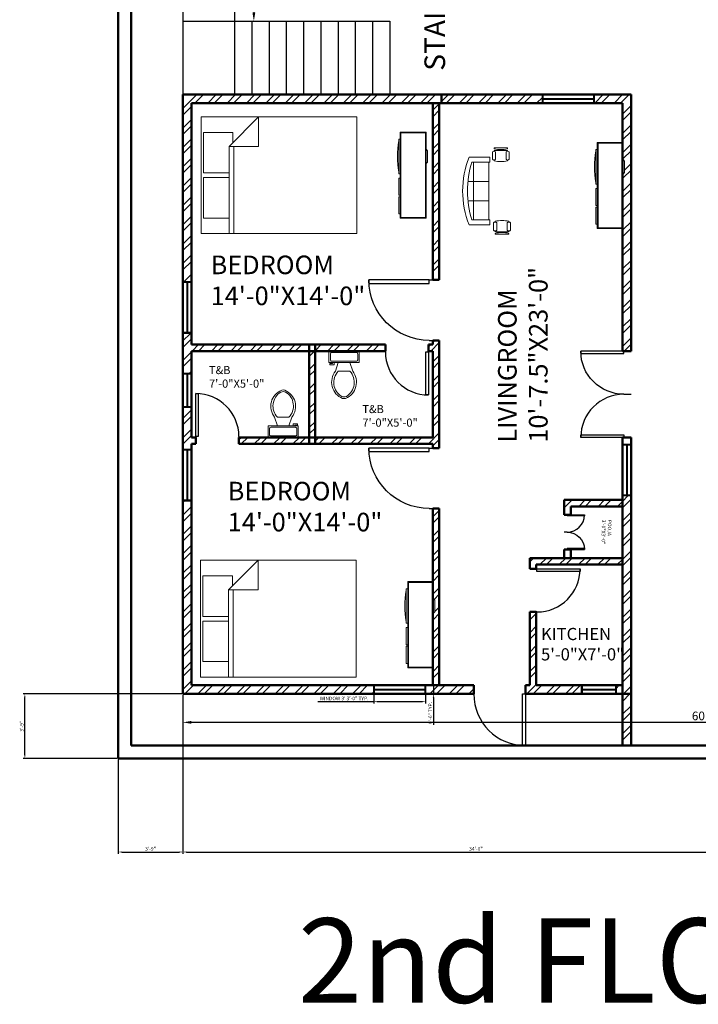
# Model space of a CAD drawing. Units: inches. Extents: x -12550 to 6516, y 1273 to 18700.
# Tile 8 of 19: x 3066 to 3538, y 1273 to 1958. Entities that reach past the tile are written whole.
import ezdxf

# ---------------------------------------------------------------- set-up
doc = ezdxf.new("R2010")
doc.units = ezdxf.units.IN
for name, color, linetype, lineweight in [('A-ANNO-DIMS', 2, 'Continuous', 18), ('A-ANNO-TEXT', 7, 'Continuous', 25), ('A-AREA-IDEN', 1, 'Continuous', 18), ('A-DOOR', 5, 'Continuous', 25), ('A-FLOR-STRS', 6, 'Continuous', 25), ('A-FURN', 8, 'Continuous', 18), ('A-GLAZ', 3, 'Continuous', 25), ('A-WALL', 7, 'Continuous', 50), ('A-WALL-PATT', 8, 'Continuous', 13)]:
    doc.layers.add(name, color=color, linetype=linetype, lineweight=lineweight)
doc.styles.get("Standard").update_dxf_attribs({"font": 'arial.ttf'})
doc.dimstyles.new('ISO-25', dxfattribs={"dimtxt": 2.5, "dimasz": 2.5, "dimexe": 1.25, "dimexo": 0.625, "dimtad": 1, "dimlunit": 4, "dimtxsty": 'Standard', "dimcen": 2.5, "dimadec": 0, "dimazin": 0, "dimtfac": 1, "dimtmove": 0, "dimatfit": 3, "dimfxl": 1, "dimarcsym": 0})
pattern_1 = [(45, (1161.5385, 0), (-6.735192, 6.735192), []), (45, (1166.029, 0), (-6.735192, 6.735192), [])]

# ---------------------------------------------------------------- blocks, each defined once
blk = doc.blocks.new('*U2')
for p, q in [((0, 0), (0, -5)), ((30, 0), (30, -5))]:
    blk.add_line(p, q)
blk.add_lwpolyline([(0, 0), (0, 30), (1.75, 30), (1.75, 0)], close=True)
blk.add_arc((0, 0), 30, 0, 90)
blk = doc.blocks.new('Bed - Queen')
for p, q in [((0, -80.00003), (0, 0)), ((0, 0), (59.99999, 0)), ((59.99999, 0), (59.99999, -80.00003)), ((7.99999, -1.2), (28.79998, -1.2)), ((7.99999, -14.4), (7.99999, -1.2)), ((28.79998, -1.2), (28.79998, -14.4)), ((31.19999, -1.2), (51.99999, -1.2)), ((31.19999, -14.4), (31.19999, -1.2)), ((51.99999, -1.2), (51.99999, -16.4)), ((0, -14.4), (44.8, -14.4)), ((59.99999, -29.6), (44.8, -14.4)), ((44.8, -14.4), (44.8, -29.6)), ((44.8, -16.8), (0, -16.8)), ((51.99999, -16.4), (46.79936, -16.4)), ((44.8, -29.6), (59.99999, -29.6)), ((59.99999, -80.00003), (0, -80.00003))]:
    blk.add_line(p, q)
blk = doc.blocks.new('Toilet - top')
for p, q in [((9.5, -6), (9.5, -2)), ((-10, -8.5), (-8, -8.5)), ((-10, -9.5), (-10, -8.5)), ((-7, -9.5), (-10, -9.5)), ((-8, -8.5), (-8, -8)), ((-7, -8), (-7, -9.5)), ((-4, -8), (-6, -14)), ((4, -8), (6, -14)), ((4, -14), (-4, -14))]:
    blk.add_line(p, q)
blk.add_lwpolyline([(10.5, -8), (10.5, 0), (-10.5, 0), (-10.5, -8)], close=True)
for points in [[(-9.5, -2), (-9.5, -6)], [(8.5, -1), (-8.5, -1)], [(-8.5, -7), (8.5, -7)]]:
    blk.add_lwpolyline(points)
for centre, radius, start, end in [((-8.62, -1.88), 0.884, 81.8699, 188.1301), ((-8.62, -6.12), 0.884, 171.8699, 278.1301), ((8.62, -1.88), 0.884, 351.8699, 98.1301), ((8.62, -6.12), 0.884, 261.8699, 8.1301), ((3.52, -21.58), 12.17, 141.46911, 247.97143), ((4.2, -21.82), 11.33, 136.36773, 238.94682), ((-3.52, -21.58), 12.17, 292.02843, 38.53071), ((-4.2, -21.82), 11.33, 301.05301, 43.63209), ((0, -27.88), 4, 245.73182, 294.26817), ((0, -29), 4, 254.86053, 285.13947)]:
    blk.add_arc(centre, radius, start, end)
blk = doc.blocks.new('Entertainment Center')
for p, q in [((-4, 0), (-5, -1)), ((4, 0), (-4, 0)), ((5, -1), (4, 0)), ((-17, -19), (-17, -1)), ((-17, -1), (43, -1)), ((-16.5, -18.5), (-16.5, -1.5)), ((-16.5, -1.5), (42.5, -1.5)), ((42.5, -1.5), (42.5, -18.5)), ((43, -1), (43, -19)), ((43, -19), (-17, -19)), ((42.5, -18.5), (-16.5, -18.5)), ((-12, -20), (-12, -19)), ((12, -20), (-12, -20)), ((12, -19), (12, -20)), ((15, -20), (15, -19)), ((27, -20), (15, -20)), ((27, -19), (27, -20)), ((28, -20), (28, -19)), ((40, -20), (28, -20)), ((40, -19), (40, -20))]:
    blk.add_line(p, q)
blk.add_arc((0, 40), 61, 259.6111, 280.3889)
blk = doc.blocks.new('Sofa - Roundback 7 ft.')
for p, q in [((-36.000027, -34), (-36.000027, -11.4696)), ((-12.00002, -32.4421), (-12.00003, -6.5971)), ((11.99997, -32.4421), (11.99998, -6.5971)), ((35.99998, -34), (35.99998, -11.4696)), ((-35.999844, -13.3819), (35.9998, -13.3819)), ((-36.000027, -32.4421), (35.99998, -32.4421))]:
    blk.add_line(p, q)
for points in [[(-36.000027, -34), (-42.000027, -34), (-42.000027, -8)], [(41.99998, -8), (41.99998, -34), (35.99998, -34)]]:
    blk.add_lwpolyline(points)
for centre, radius, start, end in [((0, -114.25), 114.25, 68.43141, 111.5686), ((-0.00001, -127.1968), 121.1968, 72.72033, 107.2797)]:
    blk.add_arc(centre, radius, start, end)
blk = doc.blocks.new('Chair - Desk')
for p, q in [((-8.5, 0), (-8.5, -1)), ((-8.5, 0), (8.5, 0)), ((8.5, 0), (8.5, -1)), ((-10.5, -5), (-10.5, -14)), ((-8.5, -3), (-8.5, -4)), ((-8.5, -3), (8.5, -3)), ((-6.5, -14), (-6.5, -5)), ((-2, -3), (-2, -1.9355)), ((2, -1.9576), (2, -3)), ((6.5, -5), (6.5, -14)), ((8.5, -3), (8.5, -4)), ((10.5, -14), (10.5, -5)), ((-8.5, -15), (-8.5, -16)), ((8.5, -15), (8.5, -16))]:
    blk.add_line(p, q)
for centre, radius, start, end in [((-8.5, -6.5), 2.5, 36.8699, 143.1301), ((0, 34.625), 36.625, 256.5803, 283.4197), ((8.5, -6.5), 2.5, 36.8699, 143.1301), ((-8.5, -12.5), 2.5, 216.8699, 323.1301), ((0, 19.625), 36.625, 256.5803, 283.4197), ((8.5, -12.5), 2.5, 216.8699, 323.1301)]:
    blk.add_arc(centre, radius, start, end)
blk = doc.blocks.new('*D36')
at = {"layer": 'A-ANNO-DIMS', "color": 0, "lineweight": -2, "transparency": 16777216}
for p, q in [((3215.85, 2008.25), (3229.9, 2008.25)), ((3228.65, 2002.25), (3228.65, 1963.25)), ((3215.85, 1957.25), (3229.9, 1957.25))]:
    blk.add_line(p, q, dxfattribs=at)
at = {"layer": 'A-ANNO-DIMS', "color": 0, "transparency": 16777216}
for points in [[(3227.65, 2002.25), (3229.65, 2002.25), (3228.65, 2008.25)], [(3227.65, 1963.25), (3229.65, 1963.25), (3228.65, 1957.25)]]:
    blk.add_solid(points, dxfattribs=at)
at = {"layer": 'Defpoints', "color": 0, "transparency": 16777216}
for p in [(3215.23, 2008.25), (3215.23, 1957.25), (3228.65, 1957.25)]:
    blk.add_point(p, dxfattribs=at)
at = {"layer": 'A-ANNO-DIMS', "color": 0, "transparency": 16777216, "insert": (3224.96, 1982.75), "char_height": 6, "attachment_point": 5, "rotation": 90}
blk.add_mtext('4\'-3"', dxfattribs=at)
blk = doc.blocks.new('*D31')
at = {"layer": 'A-ANNO-DIMS', "color": 0, "lineweight": -2, "transparency": 16777216}
for p, q in [((3179.23, 1488.62), (3179.23, 1468.21)), ((3899.23, 1488.62), (3899.23, 1468.21)), ((3893.23, 1469.46), (3185.23, 1469.46))]:
    blk.add_line(p, q, dxfattribs=at)
at = {"layer": 'A-ANNO-DIMS', "color": 0, "transparency": 16777216}
for points in [[(3185.23, 1470.46), (3185.23, 1468.46), (3179.23, 1469.46)], [(3893.23, 1470.46), (3893.23, 1468.46), (3899.23, 1469.46)]]:
    blk.add_solid(points, dxfattribs=at)
at = {"layer": 'Defpoints', "color": 0, "transparency": 16777216}
for p in [(3179.23, 1489.25), (3899.23, 1489.25), (3179.23, 1469.46)]:
    blk.add_point(p, dxfattribs=at)
at = {"layer": 'A-ANNO-DIMS', "color": 0, "transparency": 16777216, "insert": (3539.23, 1473.15), "char_height": 6, "attachment_point": 5}
blk.add_mtext("60'", dxfattribs=at)
blk = doc.blocks.new('WIN-3FT')
for p, q in [((0, 0), (0, 6)), ((0, 6), (36.02, 6)), ((36.02, 0), (0, 0)), ((0.5, 0), (0.5, 6)), ((35.52, 3.2), (0.5, 3.2)), ((35.52, 2.8), (0.5, 2.8)), ((35.52, 6), (35.52, 0)), ((36.02, 6), (36.02, 0))]:
    blk.add_line(p, q)
blk = doc.blocks.new('WIN-2FT')
for p, q in [((0, 0), (0, 24.02)), ((0, 24.02), (6, 24.02)), ((0, 23.52), (6, 23.52)), ((2.8, 0.5), (2.8, 23.52)), ((3.2, 0.5), (3.2, 23.52)), ((6, 24.02), (6, 0)), ((6, 0.5), (0, 0.5)), ((6, 0), (0, 0))]:
    blk.add_line(p, q)
blk = doc.blocks.new('*D63')
at = {"layer": 'A-ANNO-DIMS', "color": 0, "lineweight": -2, "transparency": 16777216}
for p, q in [((3312.18, 1488.62), (3312.18, 1482.59)), ((3348.2, 1488.62), (3348.2, 1482.59)), ((3312.18, 1483.84), (3273.21, 1483.84)), ((3345.7, 1483.84), (3314.68, 1483.84))]:
    blk.add_line(p, q, dxfattribs=at)
at = {"layer": 'A-ANNO-DIMS', "color": 0, "transparency": 16777216}
for points in [[(3314.68, 1484.26), (3314.68, 1483.43), (3312.18, 1483.84)], [(3345.7, 1484.26), (3345.7, 1483.43), (3348.2, 1483.84)]]:
    blk.add_solid(points, dxfattribs=at)
at = {"layer": 'Defpoints', "color": 0, "transparency": 16777216}
for p in [(3312.18, 1489.25), (3348.2, 1489.25), (3312.18, 1483.84)]:
    blk.add_point(p, dxfattribs=at)
at = {"layer": 'A-ANNO-DIMS', "color": 0, "transparency": 16777216, "insert": (3291.45, 1485.76), "char_height": 2.5, "attachment_point": 5}
blk.add_mtext('WINDOW 3\' 3\'-0" TYP.', dxfattribs=at)
blk = doc.blocks.new('*D64')
at = {"layer": 'A-ANNO-DIMS', "color": 0, "lineweight": -2, "transparency": 16777216}
for p, q in [((3348.82, 1495.25), (3354.85, 1495.25)), ((3353.6, 1497.75), (3353.6, 1500.25)), ((3353.6, 1495.25), (3353.6, 1489.25)), ((3348.82, 1489.25), (3354.85, 1489.25)), ((3353.6, 1486.75), (3353.6, 1467.76))]:
    blk.add_line(p, q, dxfattribs=at)
at = {"layer": 'A-ANNO-DIMS', "color": 0, "transparency": 16777216}
for points in [[(3353.18, 1497.75), (3354.01, 1497.75), (3353.6, 1495.25)], [(3353.18, 1486.75), (3354.01, 1486.75), (3353.6, 1489.25)]]:
    blk.add_solid(points, dxfattribs=at)
at = {"layer": 'Defpoints', "color": 0, "transparency": 16777216}
for p in [(3348.2, 1495.25), (3348.2, 1489.25), (3353.6, 1489.25)]:
    blk.add_point(p, dxfattribs=at)
at = {"layer": 'A-ANNO-DIMS', "color": 0, "transparency": 16777216, "insert": (3351.7, 1476), "char_height": 2.5, "attachment_point": 5, "rotation": 90}
blk.add_mtext('0\'-6" TYP.', dxfattribs=at)
blk = doc.blocks.new('*D105')
at = {"layer": 'A-ANNO-DIMS', "color": 0, "lineweight": -2, "transparency": 16777216}
for p, q in [((3179.23, 1488.62), (3179.23, 1378)), ((3134.23, 1443.62), (3134.23, 1378)), ((3136.73, 1379.25), (3176.73, 1379.25))]:
    blk.add_line(p, q, dxfattribs=at)
at = {"layer": 'A-ANNO-DIMS', "color": 0, "transparency": 16777216}
for points in [[(3136.73, 1379.66), (3136.73, 1378.83), (3134.23, 1379.25)], [(3176.73, 1379.66), (3176.73, 1378.83), (3179.23, 1379.25)]]:
    blk.add_solid(points, dxfattribs=at)
at = {"layer": 'Defpoints', "color": 0, "transparency": 16777216}
for p in [(3179.23, 1489.25), (3134.23, 1444.25), (3179.23, 1379.25)]:
    blk.add_point(p, dxfattribs=at)
at = {"layer": 'A-ANNO-DIMS', "color": 0, "transparency": 16777216, "insert": (3156.73, 1381.15), "char_height": 2.5, "attachment_point": 5}
blk.add_mtext('3\'-9"', dxfattribs=at)
blk = doc.blocks.new('*D106')
at = {"layer": 'A-ANNO-DIMS', "color": 0, "lineweight": -2, "transparency": 16777216}
for p, q in [((3179.23, 1488.62), (3179.23, 1378)), ((3587.23, 1488.62), (3587.23, 1378)), ((3181.73, 1379.25), (3584.73, 1379.25))]:
    blk.add_line(p, q, dxfattribs=at)
at = {"layer": 'A-ANNO-DIMS', "color": 0, "transparency": 16777216}
for points in [[(3181.73, 1379.66), (3181.73, 1378.83), (3179.23, 1379.25)], [(3584.73, 1379.66), (3584.73, 1378.83), (3587.23, 1379.25)]]:
    blk.add_solid(points, dxfattribs=at)
at = {"layer": 'Defpoints', "color": 0, "transparency": 16777216}
for p in [(3179.23, 1489.25), (3587.23, 1489.25), (3587.23, 1379.25)]:
    blk.add_point(p, dxfattribs=at)
at = {"layer": 'A-ANNO-DIMS', "color": 0, "transparency": 16777216, "insert": (3383.23, 1381.15), "char_height": 2.5, "attachment_point": 5}
blk.add_mtext('34\'-0"', dxfattribs=at)
blk = doc.blocks.new('*D110')
at = {"layer": 'A-ANNO-DIMS', "color": 0, "lineweight": -2, "transparency": 16777216}
for p, q in [((3178.6, 1489.25), (3067.98, 1489.25)), ((3069.23, 1446.75), (3069.23, 1486.75)), ((3133.6, 1444.25), (3067.98, 1444.25))]:
    blk.add_line(p, q, dxfattribs=at)
at = {"layer": 'A-ANNO-DIMS', "color": 0, "transparency": 16777216}
for points in [[(3068.81, 1486.75), (3069.64, 1486.75), (3069.23, 1489.25)], [(3068.81, 1446.75), (3069.64, 1446.75), (3069.23, 1444.25)]]:
    blk.add_solid(points, dxfattribs=at)
at = {"layer": 'Defpoints', "color": 0, "transparency": 16777216}
for p in [(3069.23, 1489.25), (3179.23, 1489.25), (3134.23, 1444.25)]:
    blk.add_point(p, dxfattribs=at)
at = {"layer": 'A-ANNO-DIMS', "color": 0, "transparency": 16777216, "insert": (3067.33, 1466.75), "char_height": 2.5, "attachment_point": 5, "rotation": 90}
blk.add_mtext('3\'-9"', dxfattribs=at)

msp = doc.modelspace()

# ---------------------------------------------------------------- hatches: boundary and pattern name
at = {"layer": 'A-WALL-PATT'}
h = msp.add_hatch(dxfattribs=at)
h.set_pattern_fill('ANSI32', color=256)
h.set_pattern_definition(pattern_1)
h.paths.add_polyline_path([(3185.227, 1900.247), (3359.227, 1900.247), (3359.227, 1906.247), (3179.227, 1906.247), (3179.227, 1776.138), (3185.227, 1776.138)])
h = msp.add_hatch(dxfattribs=at)
h.set_pattern_fill('ANSI32', color=256)
h.set_pattern_definition(pattern_1)
h.paths.add_polyline_path([(3429.479, 1906.247), (3359.227, 1906.247), (3359.227, 1900.247), (3429.479, 1900.247)])
h = msp.add_hatch(dxfattribs=at)
h.set_pattern_fill('ANSI32', color=256)
h.set_pattern_definition(pattern_1)
h.paths.add_polyline_path([(3491.227, 1906.247), (3465.496, 1906.247), (3465.496, 1900.247), (3485.227, 1900.247), (3485.227, 1872.972), (3485.727, 1872.972), (3485.727, 1860.972), (3486.727, 1859.972), (3486.727, 1851.972), (3485.727, 1850.972), (3485.727, 1812.972), (3485.227, 1727.747), (3486.227, 1727.747), (3491.227, 1727.747)])
h = msp.add_hatch(dxfattribs=at)
h.set_pattern_fill('ANSI32', color=256)
h.set_pattern_definition(pattern_1)
h.paths.add_polyline_path([(3357.727, 1900.247), (3353.227, 1900.247), (3353.227, 1777.247), (3357.727, 1777.247)], flags=17)
h = msp.add_hatch(dxfattribs=at)
h.set_pattern_fill('ANSI32', color=256)
h.set_pattern_definition(pattern_1)
h.paths.add_polyline_path([(3267.227, 1732.247), (3185.227, 1732.247), (3185.227, 1740.121), (3179.227, 1740.121), (3179.227, 1712.466), (3185.227, 1712.466), (3185.227, 1727.747), (3267.227, 1727.747)])
h = msp.add_hatch(dxfattribs=at)
h.set_pattern_fill('ANSI32', color=256)
h.set_pattern_definition(pattern_1)
h.paths.add_polyline_path([(3357.727, 1735.247), (3353.227, 1735.247), (3353.227, 1732.247), (3350.227, 1732.247), (3350.227, 1727.747), (3353.227, 1727.747), (3353.227, 1667.747), (3271.227, 1667.747), (3271.227, 1663.247), (3353.227, 1663.247), (3353.227, 1660.247), (3357.727, 1660.247)])
h = msp.add_hatch(dxfattribs=at)
h.set_pattern_fill('ANSI32', color=256)
h.set_pattern_definition(pattern_1)
h.paths.add_polyline_path([(3271.227, 1727.747), (3267.227, 1727.747), (3267.227, 1667.747), (3271.227, 1667.747)])
h = msp.add_hatch(dxfattribs=at)
h.set_pattern_fill('ANSI32', color=256)
h.set_pattern_definition(pattern_1)
h.paths.add_polyline_path([(3320.227, 1732.247), (3271.227, 1732.247), (3271.227, 1727.747), (3320.227, 1727.747)], flags=17)
h = msp.add_hatch(dxfattribs=at)
h.set_pattern_fill('ANSI32', color=256)
h.set_pattern_definition(pattern_1)
h.paths.add_polyline_path([(3185.227, 1688.449), (3179.227, 1688.449), (3179.227, 1659.453), (3185.227, 1659.453), (3185.227, 1663.247), (3188.227, 1663.247), (3188.227, 1667.747), (3185.227, 1667.747)])
h = msp.add_hatch(dxfattribs=at)
h.set_pattern_fill('ANSI32', color=256)
h.set_pattern_definition(pattern_1)
h.paths.add_polyline_path([(3267.227, 1667.747), (3218.227, 1667.747), (3218.227, 1663.247), (3267.227, 1663.247)])
h = msp.add_hatch(dxfattribs=at)
h.set_pattern_fill('ANSI32', color=256)
h.set_pattern_definition(pattern_1)
h.paths.add_polyline_path([(3485.227, 1624.247), (3444.727, 1624.247), (3444.727, 1613.747), (3446.727, 1613.747), (3449.227, 1613.747), (3449.227, 1619.747), (3485.227, 1619.747)])
h = msp.add_hatch(dxfattribs=at)
h.set_pattern_fill('ANSI32', color=256)
h.set_pattern_definition(pattern_1)
h.paths.add_polyline_path([(3491.227, 1627.032), (3485.227, 1627.032), (3485.227, 1495.247), (3480.833, 1495.247), (3480.833, 1489.247), (3491.227, 1489.247)])
h = msp.add_hatch(dxfattribs=at)
h.set_pattern_fill('ANSI32', color=256)
h.set_pattern_definition(pattern_1)
h.paths.add_polyline_path([(3185.227, 1623.435), (3179.227, 1623.435), (3179.227, 1489.247), (3312.178, 1489.247), (3312.178, 1495.247), (3185.227, 1495.247)])
h = msp.add_hatch(dxfattribs=at)
h.set_pattern_fill('ANSI32', color=256)
h.set_pattern_definition(pattern_1)
h.paths.add_polyline_path([(3357.727, 1618.247), (3353.227, 1618.247), (3353.227, 1567.365), (3353.727, 1567.365), (3353.727, 1555.365), (3354.727, 1554.365), (3354.727, 1546.365), (3353.727, 1545.365), (3353.727, 1507.365), (3353.227, 1495.247), (3357.727, 1495.247)])
h = msp.add_hatch(dxfattribs=at)
h.set_pattern_fill('ANSI32', color=256)
h.set_pattern_definition(pattern_1)
h.paths.add_polyline_path([(3485.227, 1583.747), (3420.727, 1583.747), (3420.727, 1576.247), (3425.227, 1576.247), (3425.227, 1579.247), (3485.227, 1579.247)])
h = msp.add_hatch(dxfattribs=at)
h.set_pattern_fill('ANSI32', color=256)
h.set_pattern_definition(pattern_1)
h.paths.add_polyline_path([(3456.815, 1495.247), (3425.227, 1495.247), (3425.227, 1546.247), (3420.727, 1546.247), (3420.727, 1495.247), (3417.727, 1495.247), (3417.727, 1489.247), (3456.815, 1489.247)])
h = msp.add_hatch(dxfattribs=at)
h.set_pattern_fill('ANSI32', color=256)
h.set_pattern_definition(pattern_1)
h.paths.add_polyline_path([(3381.727, 1495.247), (3348.196, 1495.247), (3348.196, 1489.247), (3381.727, 1489.247)])
h = msp.add_hatch(dxfattribs=at)
h.set_pattern_fill('ANSI32', color=256)
h.set_pattern_definition(pattern_1)
h.paths.add_polyline_path([(3491.227, 1489.247), (3485.227, 1489.247), (3485.227, 1453.247), (3491.227, 1453.247)])

# ---------------------------------------------------------------- linework, layer by layer
at = {"layer": 'A-FLOR-STRS'}
for p, q in [((3179.227, 2056.247), (3179.227, 1906.247)), ((3215.227, 2056.247), (3215.227, 1906.247)), ((3179.227, 1957.247), (3323.227, 1957.247)), ((3227.227, 1957.247), (3227.227, 1906.247)), ((3239.227, 1957.247), (3239.227, 1906.247)), ((3251.227, 1957.247), (3251.227, 1906.247)), ((3263.227, 1957.247), (3263.227, 1906.247)), ((3275.227, 1957.247), (3275.227, 1906.247)), ((3287.227, 1957.247), (3287.227, 1906.247)), ((3299.227, 1957.247), (3299.227, 1906.247)), ((3311.227, 1957.247), (3311.227, 1906.247)), ((3323.227, 1957.247), (3323.227, 1906.247)), ((3179.227, 1906.247), (3359.227, 1906.247))]:
    msp.add_line(p, q, dxfattribs=at)
at = {"layer": 'A-WALL'}
for p, q in [((3134.227, 1444.247), (3134.227, 2518.247)), ((3143.227, 1453.247), (3143.227, 2509.247)), ((3491.227, 1906.247), (3179.227, 1906.247)), ((3179.227, 1489.247), (3179.227, 1906.247)), ((3359.227, 1900.247), (3359.227, 1906.247)), ((3491.227, 1727.747), (3491.227, 1906.247)), ((3485.227, 1900.247), (3185.227, 1900.247)), ((3185.227, 1732.247), (3185.227, 1900.247)), ((3353.227, 1777.247), (3353.227, 1900.247)), ((3357.727, 1777.247), (3357.727, 1900.247)), ((3485.227, 1727.747), (3485.227, 1900.247)), ((3357.727, 1777.247), (3353.227, 1777.247)), ((3353.227, 1732.247), (3353.227, 1735.247)), ((3353.227, 1732.247), (3353.227, 1735.247)), ((3353.227, 1735.247), (3357.727, 1735.247)), ((3357.727, 1660.247), (3357.727, 1735.247)), ((3320.227, 1732.247), (3185.227, 1732.247)), ((3320.227, 1727.747), (3185.227, 1727.747)), ((3185.227, 1667.747), (3185.227, 1727.747)), ((3267.227, 1663.247), (3267.227, 1732.247)), ((3271.227, 1663.247), (3271.227, 1732.247)), ((3320.227, 1727.747), (3320.227, 1732.247)), ((3353.227, 1732.247), (3350.227, 1732.247)), ((3353.227, 1732.247), (3350.227, 1732.247)), ((3350.227, 1732.247), (3350.227, 1727.747)), ((3353.227, 1727.747), (3350.227, 1727.747)), ((3353.227, 1667.747), (3353.227, 1727.747)), ((3491.227, 1727.747), (3485.227, 1727.747)), ((3188.227, 1667.747), (3185.227, 1667.747)), ((3188.227, 1663.247), (3188.227, 1667.747)), ((3353.227, 1667.747), (3218.227, 1667.747)), ((3218.227, 1667.747), (3353.227, 1667.747)), ((3218.227, 1667.747), (3218.227, 1663.247)), ((3491.227, 1667.747), (3485.227, 1667.747)), ((3485.227, 1453.247), (3485.227, 1667.747)), ((3491.227, 1489.247), (3491.227, 1667.747)), ((3188.227, 1663.247), (3185.227, 1663.247)), ((3185.227, 1495.247), (3185.227, 1663.247)), ((3185.227, 1663.247), (3188.227, 1663.247)), ((3353.227, 1663.247), (3218.227, 1663.247)), ((3353.227, 1660.247), (3353.227, 1663.247)), ((3357.727, 1660.247), (3353.227, 1660.247)), ((3357.727, 1663.247), (3357.727, 1660.247)), ((3485.227, 1624.247), (3444.727, 1624.247)), ((3444.727, 1613.747), (3444.727, 1624.247)), ((3353.227, 1495.247), (3353.227, 1618.247)), ((3353.227, 1618.247), (3357.727, 1618.247)), ((3357.727, 1495.247), (3357.727, 1618.247)), ((3485.227, 1619.747), (3449.227, 1619.747)), ((3449.227, 1613.747), (3449.227, 1619.747)), ((3444.727, 1613.747), (3449.227, 1613.747)), ((3444.727, 1583.747), (3444.727, 1589.747)), ((3449.227, 1589.747), (3444.727, 1589.747)), ((3449.227, 1583.747), (3449.227, 1589.747)), ((3449.227, 1583.747), (3449.227, 1589.747)), ((3485.227, 1583.747), (3420.727, 1583.747)), ((3420.727, 1576.247), (3420.727, 1583.747)), ((3444.727, 1583.747), (3444.727, 1588.747)), ((3425.227, 1576.247), (3420.727, 1576.247)), ((3485.227, 1579.247), (3425.227, 1579.247)), ((3425.227, 1576.247), (3425.227, 1579.247)), ((3425.227, 1579.247), (3425.227, 1576.247)), ((3420.727, 1495.247), (3420.727, 1546.247)), ((3420.727, 1546.247), (3425.227, 1546.247)), ((3425.227, 1495.247), (3425.227, 1546.247)), ((3381.727, 1495.247), (3185.227, 1495.247)), ((3381.727, 1495.247), (3357.727, 1495.247)), ((3381.727, 1489.247), (3381.727, 1495.247)), ((3420.727, 1495.247), (3417.727, 1495.247)), ((3420.727, 1495.247), (3417.727, 1495.247)), ((3417.727, 1495.247), (3417.727, 1489.247)), ((3485.227, 1495.247), (3425.227, 1495.247)), ((3381.727, 1489.247), (3179.227, 1489.247)), ((3491.227, 1489.247), (3417.727, 1489.247)), ((3491.227, 1489.247), (3491.227, 1453.247)), ((3143.227, 1453.247), (3935.227, 1453.247)), ((3681.727, 1453.247), (3417.727, 1453.247)), ((3134.227, 1444.247), (3944.227, 1444.247))]:
    msp.add_line(p, q, dxfattribs=at)

# ---------------------------------------------------------------- block references
at = {"layer": 'A-DOOR'}
for p, xscale, yscale, zscale, rotation in [((3350.727, 1777.247), -1.4, 1.4, 1.4, 90), ((3350.727, 1660.247), -1.4, 1.4, 1.4, 90), ((3446.727, 1613.747), 0.399999999999997, 0.399999999999997, 0.399999999999997, 270), ((3446.727, 1589.747), -0.399999999999997, 0.399999999999997, 0.399999999999997, 270), ((3417.727, 1489.247), 1.199999999999999, 1.199999999999999, 1.199999999999999, 180)]:
    msp.add_blockref('*U2', p, dxfattribs=dict(at, xscale=xscale, yscale=yscale, zscale=zscale, rotation=rotation))
for p, rotation in [((3350.227, 1727.247), 180), ((3486.227, 1667.747), 90), ((3425.727, 1576.247), 270)]:
    msp.add_blockref('*U2', p, dxfattribs=dict(at, rotation=rotation))
at = {"layer": 'A-DOOR', "xscale": -1, "rotation": 90}
msp.add_blockref('*U2', (3486.227, 1727.747), dxfattribs=at)
at = {"layer": 'A-DOOR'}
msp.add_blockref('*U2', (3188.227, 1668.247), dxfattribs=at)
at = {"layer": 'A-FURN'}
for name, p, xscale, yscale, zscale, rotation in [('Bed - Queen', (3191.878, 1809.493), 1.354827908062564, 1.354827908062564, 1.354827908062564, 90), ('Sofa - Roundback 7 ft.', (3373.986, 1839.138), 0.5595223685495907, 0.5595223685495907, 0.5595223685495907, 90), ('Chair - Desk', (3401.426, 1809.138), 0.5595223685495907, 0.5595223685495907, 0.5595223685495907, 180), ('Bed - Queen', (3191.576, 1500.915), 1.354827908062564, 1.354827908062564, 1.354827908062564, 90)]:
    msp.add_blockref(name, p, dxfattribs=dict(at, xscale=xscale, yscale=yscale, zscale=zscale, rotation=rotation))
for name, p, rotation in [('Entertainment Center', (3349.568, 1863.204), 270), ('Entertainment Center', (3486.727, 1855.972), 270), ('Toilet - top', (3249.075, 1667.747), 180), ('Entertainment Center', (3354.727, 1550.365), 270)]:
    msp.add_blockref(name, p, dxfattribs=dict(at, rotation=rotation))
at = {"layer": 'A-FURN', "xscale": 0.5595223685495907, "yscale": 0.5595223685495907, "zscale": 0.5595223685495907}
msp.add_blockref('Chair - Desk', (3400.572, 1869.122), dxfattribs=at)
at = {"layer": 'A-FURN'}
msp.add_blockref('Toilet - top', (3291.439, 1727.747), dxfattribs=at)
at = {"layer": 'A-GLAZ'}
for name, p, rotation in [('WIN-3FT', (3465.496, 1906.247), 180), ('WIN-3FT', (3185.228, 1740.121), 90.00000000000175), ('WIN-2FT', (3185.227, 1712.467), 180), ('WIN-3FT', (3185.228, 1623.436), 90.00000000000163), ('WIN-3FT', (3491.228, 1627.032), 89.9999999999992), ('WIN-3FT', (3348.195, 1495.247), 180), ('WIN-2FT', (3456.815, 1495.247), 269.9999999999929)]:
    msp.add_blockref(name, p, dxfattribs=dict(at, rotation=rotation))

# ---------------------------------------------------------------- texts
at = {"layer": 'A-ANNO-TEXT', "insert": (3259.388, 1333.138), "char_height": 58.816, "attachment_point": 1}
msp.add_mtext('2nd FLOOR', dxfattribs=at)
at = {"layer": 'A-AREA-IDEN', "attachment_point": 1}
for s, width, gutter_width, insert, char_height, rotation in [('STAIRCASE', 2.19144, 71.795, (3347.404, 1922.837), 14.3589, 90), ('POOJA\\P3\'-0"X3\'-0"', 0.78585, 12.5, (3477.604, 1610.304), 2.5, 269.183853)]:
    msp.add_mtext_dynamic_manual_height_columns(s, width=width, gutter_width=gutter_width, heights=[0], dxfattribs=dict(at, insert=insert, char_height=char_height, rotation=rotation))
at = {"layer": 'A-AREA-IDEN', "char_height": 12.93169, "attachment_point": 1}
for insert in [(3198.564, 1794.217), (3210.445, 1636.812)]:
    msp.add_mtext('BEDROOM\\P14\'-0"X14\'-0"', dxfattribs=dict(at, insert=insert))
at = {"layer": 'A-AREA-IDEN', "insert": (3398.633, 1664.034), "char_height": 12.93169, "attachment_point": 1, "rotation": 90}
msp.add_mtext('LIVINGROOM\\P10\'-7.5"X23\'-0"', dxfattribs=at)
at = {"layer": 'A-AREA-IDEN', "attachment_point": 1}
for s, width, gutter_width, insert, char_height in [('T&B\\P7\'-0"X5\'-0"', 4.19569, 28.328, (3197.403, 1717.416), 5.66556), ('T&B\\P7\'-0"X5\'-0"', 4.19569, 28.328, (3304.165, 1690.282), 5.66556), ('KITCHEN\\P5\'-0"X7\'-0"', 1.29487, 42.422, (3428.549, 1535.176), 8.48435)]:
    msp.add_mtext_dynamic_manual_height_columns(s, width=width, gutter_width=gutter_width, heights=[0], dxfattribs=dict(at, insert=insert, char_height=char_height))

# ---------------------------------------------------------------- dimensions: what is measured, and where the dimension line sits
at = {"layer": 'A-ANNO-DIMS'}
for base, p1, p2, override, picture, middle in [((3228.649, 1957.247), (3215.227, 2008.247), (3215.227, 1957.247), {"dimtxt": 6, "dimasz": 6, "dimclrd": 0, "dimclre": 0, "dimclrt": 0}, '*D36', (3224.959, 1982.747)), ((3069.227, 1489.247), (3134.227, 1444.247), (3179.227, 1489.247), {"dimdec": 1, "dimlfac": 1, "dimrnd": 0, "dimzin": 1, "dimdsep": 46, "dimlunit": 4, "dimfrac": 2}, '*D110', (3067.325, 1466.747))]:
    dim = msp.add_linear_dim(base=base, p1=p1, p2=p2, angle=90, dimstyle='ISO-25', override=override, dxfattribs=at)
    dim.commit()
    dim.dimension.update_dxf_attribs({"geometry": picture, "text_midpoint": middle})
for base, p1, p2, angle, text, picture, middle in [((3312.178, 1483.845), (3348.196, 1489.247), (3312.178, 1489.247), 180, "WINDOW 3' <> TYP.", '*D63', (3291.446, 1485.764)), ((3353.598, 1489.247), (3348.196, 1495.247), (3348.196, 1489.247), 270, '<> TYP.', '*D64', (3351.697, 1476.003))]:
    dim = msp.add_linear_dim(base=base, p1=p1, p2=p2, angle=angle, text=text, dimstyle='ISO-25', override={"dimdec": 1, "dimrnd": 0, "dimzin": 1, "dimlunit": 4, "dimfrac": 2}, dxfattribs=at)
    dim.commit()
    dim.dimension.update_dxf_attribs({"geometry": picture, "text_midpoint": middle})
for base, p1, p2, override, picture, middle in [((3179.227, 1379.247), (3134.227, 1444.247), (3179.227, 1489.247), {"dimdec": 1, "dimlfac": 1, "dimrnd": 0, "dimzin": 1, "dimdsep": 46, "dimlunit": 4, "dimfrac": 2}, '*D105', (3156.727, 1381.15)), ((3179.227, 1469.461), (3899.227, 1489.247), (3179.227, 1489.247), {"dimtxt": 6, "dimasz": 6, "dimclrd": 0, "dimclre": 0, "dimclrt": 0}, '*D31', (3539.227, 1473.15)), ((3587.227, 1379.247), (3179.227, 1489.247), (3587.227, 1489.247), {"dimdec": 1, "dimlfac": 1, "dimrnd": 0, "dimzin": 1, "dimdsep": 46, "dimlunit": 4, "dimfrac": 2}, '*D106', (3383.227, 1381.15))]:
    dim = msp.add_linear_dim(base=base, p1=p1, p2=p2, dimstyle='ISO-25', override=override, dxfattribs=at)
    dim.commit()
    dim.dimension.update_dxf_attribs({"geometry": picture, "text_midpoint": middle})

doc.saveas('drawing.dxf')
